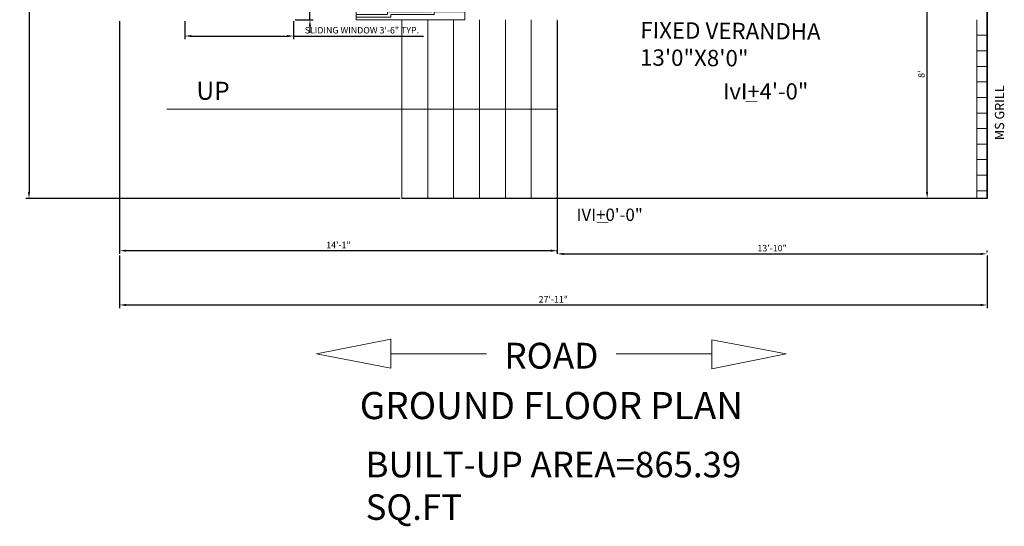
# Model space of a CAD drawing. Units: inches. Extents: x 918 to 1328, y 603 to 1174.
# Tile 1 of 4: x 918 to 1298, y 603 to 798. Entities that reach past the tile are written whole.
import ezdxf

# ---------------------------------------------------------------- set-up
doc = ezdxf.new("R2010")
doc.units = ezdxf.units.IN
for name, color, linetype, lineweight in [('A-ANNO-DIMS', 1, 'Continuous', 18), ('A-ANNO-SYMB', 1, 'Continuous', 18), ('A-ANNO-TEXT', 7, 'Continuous', 18), ('A-ANNO-TITL', 7, 'Continuous', 25), ('A-FLOR', 7, 'Continuous', 25), ('A-FLOR-RAIL', 7, 'Continuous', 18), ('A-GLAZ', 4, 'Continuous', 18), ('A-WALL', 7, 'Continuous', 35)]:
    doc.layers.add(name, color=color, linetype=linetype, lineweight=lineweight)
doc.layers.add('A-AREA-IDEN', color=251, linetype='Continuous', lineweight=20, true_color=0x636466)
doc.layers.add('A-FLOR-STRS', color=251, linetype='Continuous', lineweight=20, true_color=0x636466)
doc.styles.get("Standard").update_dxf_attribs({"font": 'arial.ttf'})
doc.dimstyles.new('ISO-25', dxfattribs={"dimtxt": 2.5, "dimasz": 2.5, "dimexe": 1.25, "dimexo": 0.625, "dimtad": 1, "dimdec": 0, "dimlunit": 3, "dimtxsty": 'Standard', "dimcen": 2.5, "dimadec": 0, "dimazin": 0, "dimtfac": 1, "dimtdec": 0, "dimtmove": 0, "dimatfit": 3, "dimfxl": 1, "dimarcsym": 0})

# ---------------------------------------------------------------- blocks, each defined once
blk = doc.blocks.new('*D11')
at = {"layer": 'A-ANNO-DIMS', "color": 0, "lineweight": -2, "transparency": 16777216}
for p, q in [((956.48, 797.62), (956.48, 707.87)), ((1125.48, 797.62), (1125.48, 707.87)), ((958.98, 709.12), (1122.98, 709.12))]:
    blk.add_line(p, q, dxfattribs=at)
at = {"layer": 'A-ANNO-DIMS', "color": 0, "transparency": 16777216}
for points in [[(958.98, 709.53), (958.98, 708.7), (956.48, 709.12)], [(1122.98, 709.53), (1122.98, 708.7), (1125.48, 709.12)]]:
    blk.add_solid(points, dxfattribs=at)
at = {"layer": 'Defpoints', "color": 0, "transparency": 16777216}
for p in [(956.48, 798.24), (1125.48, 798.24), (1125.48, 709.12)]:
    blk.add_point(p, dxfattribs=at)
at = {"layer": 'A-ANNO-DIMS', "color": 0, "transparency": 16777216, "insert": (1040.98, 711), "char_height": 2.5, "attachment_point": 5}
blk.add_mtext('14\'-1"', dxfattribs=at)
blk = doc.blocks.new('*D19')
at = {"layer": 'A-ANNO-DIMS', "color": 0, "lineweight": -2, "transparency": 16777216}
for p, q in [((956.48, 707.24), (956.48, 686.91)), ((1291.48, 707.24), (1291.48, 686.91)), ((958.98, 688.16), (1288.98, 688.16))]:
    blk.add_line(p, q, dxfattribs=at)
at = {"layer": 'A-ANNO-DIMS', "color": 0, "transparency": 16777216}
for points in [[(958.98, 688.58), (958.98, 687.74), (956.48, 688.16)], [(1288.98, 688.58), (1288.98, 687.74), (1291.48, 688.16)]]:
    blk.add_solid(points, dxfattribs=at)
at = {"layer": 'Defpoints', "color": 0, "transparency": 16777216}
for p in [(956.48, 707.87), (1291.48, 707.87), (1291.48, 688.16)]:
    blk.add_point(p, dxfattribs=at)
at = {"layer": 'A-ANNO-DIMS', "color": 0, "transparency": 16777216, "insert": (1123.98, 690.04), "char_height": 2.5, "attachment_point": 5}
blk.add_mtext('27\'-11"', dxfattribs=at)
blk = doc.blocks.new('*D20')
at = {"layer": 'A-ANNO-DIMS', "color": 0, "lineweight": -2, "transparency": 16777216}
for p, q in [((1272.05, 825.24), (1267.09, 825.24)), ((1268.34, 731.74), (1268.34, 822.74)), ((1272.05, 729.24), (1267.09, 729.24))]:
    blk.add_line(p, q, dxfattribs=at)
at = {"layer": 'A-ANNO-DIMS', "color": 0, "transparency": 16777216}
for points in [[(1267.92, 822.74), (1268.75, 822.74), (1268.34, 825.24)], [(1267.92, 731.74), (1268.75, 731.74), (1268.34, 729.24)]]:
    blk.add_solid(points, dxfattribs=at)
at = {"layer": 'Defpoints', "color": 0, "transparency": 16777216}
for p in [(1268.34, 825.24), (1272.68, 825.24), (1272.68, 729.24)]:
    blk.add_point(p, dxfattribs=at)
at = {"layer": 'A-ANNO-DIMS', "color": 0, "transparency": 16777216, "insert": (1266.44, 777.24), "char_height": 2.5, "attachment_point": 5, "rotation": 90}
blk.add_mtext("8'", dxfattribs=at)
blk = doc.blocks.new('*D21')
at = {"layer": 'A-ANNO-DIMS', "color": 0, "lineweight": -2, "transparency": 16777216}
for p, q in [((1125.48, 708.49), (1125.48, 709.12)), ((1127.98, 707.87), (1288.98, 707.87)), ((1291.48, 708.49), (1291.48, 709.12))]:
    blk.add_line(p, q, dxfattribs=at)
at = {"layer": 'A-ANNO-DIMS', "color": 0, "transparency": 16777216}
for points in [[(1127.98, 708.28), (1127.98, 707.45), (1125.48, 707.87)], [(1288.98, 708.28), (1288.98, 707.45), (1291.48, 707.87)]]:
    blk.add_solid(points, dxfattribs=at)
at = {"layer": 'Defpoints', "color": 0, "transparency": 16777216}
for p in [(1125.48, 707.87), (1291.48, 707.87), (1291.48, 707.87)]:
    blk.add_point(p, dxfattribs=at)
at = {"layer": 'A-ANNO-DIMS', "color": 0, "transparency": 16777216, "insert": (1208.48, 709.77), "char_height": 2.5, "attachment_point": 5}
blk.add_mtext('13\'-10"', dxfattribs=at)
blk = doc.blocks.new('WIN-SLIDING-42')
for p, q in [((0, 5), (0, 0)), ((42, 5), (0, 5)), ((29.09, 3), (29.09, 4.02)), ((29.09, 4.02), (42, 4.02)), ((42, 0), (42, 5)), ((0, 1.97), (12.14, 1.97)), ((0, 0.97), (13.35, 0.97)), ((0, 0), (42, 0)), ((12.14, 3), (29.09, 3)), ((12.14, 1.97), (12.14, 3)), ((13.35, 0.97), (13.35, 1.97)), ((13.35, 1.97), (30.11, 1.97)), ((30.11, 1.97), (30.11, 3)), ((30.11, 3), (42, 3))]:
    blk.add_line(p, q)
blk = doc.blocks.new('ARROW-ROAD')
for p, q in [((65.62, 5.76), (36.95, 11.23)), ((36.95, 11.23), (36.95, 0)), ((0, 5.76), (36.95, 5.76)), ((36.95, 0), (65.62, 5.76))]:
    blk.add_line(p, q)
blk = doc.blocks.new('*D32')
at = {"layer": 'A-ANNO-DIMS', "color": 0, "lineweight": -2, "transparency": 16777216}
for p, q in [((981.69, 797.62), (981.69, 790.69)), ((1023.69, 797.62), (1023.69, 790.69)), ((984.19, 791.94), (1021.19, 791.94)), ((1023.69, 791.94), (1073.9, 791.94))]:
    blk.add_line(p, q, dxfattribs=at)
at = {"layer": 'A-ANNO-DIMS', "color": 0, "transparency": 16777216}
for points in [[(984.19, 792.36), (984.19, 791.53), (981.69, 791.94)], [(1021.19, 792.36), (1021.19, 791.53), (1023.69, 791.94)]]:
    blk.add_solid(points, dxfattribs=at)
at = {"layer": 'Defpoints', "color": 0, "transparency": 16777216}
for p in [(981.69, 798.24), (1023.69, 798.24), (1023.69, 791.94)]:
    blk.add_point(p, dxfattribs=at)
at = {"layer": 'A-ANNO-DIMS', "color": 0, "transparency": 16777216, "insert": (1050.05, 793.86), "char_height": 2.5, "attachment_point": 5}
blk.add_mtext('SLIDING WINDOW 3\'-6" TYP.', dxfattribs=at)
blk = doc.blocks.new('*D33')
at = {"layer": 'A-ANNO-DIMS', "color": 0, "lineweight": -2, "transparency": 16777216}
for p, q in [((1029.99, 805.74), (1029.99, 824.73)), ((1024.31, 803.24), (1031.24, 803.24)), ((1029.99, 798.24), (1029.99, 803.24)), ((1024.31, 798.24), (1031.24, 798.24)), ((1029.99, 795.74), (1029.99, 793.24))]:
    blk.add_line(p, q, dxfattribs=at)
at = {"layer": 'A-ANNO-DIMS', "color": 0, "transparency": 16777216}
for points in [[(1029.57, 805.74), (1030.41, 805.74), (1029.99, 803.24)], [(1029.57, 795.74), (1030.41, 795.74), (1029.99, 798.24)]]:
    blk.add_solid(points, dxfattribs=at)
at = {"layer": 'Defpoints', "color": 0, "transparency": 16777216}
for p in [(1023.69, 803.24), (1029.99, 803.24), (1023.69, 798.24)]:
    blk.add_point(p, dxfattribs=at)
at = {"layer": 'A-ANNO-DIMS', "color": 0, "transparency": 16777216, "insert": (1028.09, 816.49), "char_height": 2.5, "attachment_point": 5, "rotation": 90}
blk.add_mtext('0\'-5" TYP.', dxfattribs=at)
blk = doc.blocks.new('*D44')
at = {"layer": 'A-ANNO-DIMS', "color": 0, "lineweight": -2, "transparency": 16777216}
for p, q in [((955.86, 1136.24), (920.25, 1136.24)), ((921.5, 1133.74), (921.5, 731.74)), ((1064.86, 729.24), (920.25, 729.24))]:
    blk.add_line(p, q, dxfattribs=at)
at = {"layer": 'A-ANNO-DIMS', "color": 0, "transparency": 16777216}
for points in [[(921.09, 1133.74), (921.92, 1133.74), (921.5, 1136.24)], [(921.09, 731.74), (921.92, 731.74), (921.5, 729.24)]]:
    blk.add_solid(points, dxfattribs=at)
at = {"layer": 'Defpoints', "color": 0, "transparency": 16777216}
for p in [(956.48, 1136.24), (921.5, 729.24), (1065.48, 729.24)]:
    blk.add_point(p, dxfattribs=at)
at = {"layer": 'A-ANNO-DIMS', "color": 0, "transparency": 16777216, "insert": (919.6, 932.74), "char_height": 2.5, "attachment_point": 5, "rotation": 90}
blk.add_mtext('33\'-11"', dxfattribs=at)

msp = doc.modelspace()

# ---------------------------------------------------------------- linework, layer by layer
at = {"layer": 'A-ANNO-SYMB'}
for p, q in [((1198.32, 766.78), (1202.69, 766.67)), ((1125.48, 763.74), (974.75, 763.74)), ((1140.75, 720.11), (1145.12, 720.01))]:
    msp.add_line(p, q, dxfattribs=at)
at = {"layer": 'A-FLOR'}
msp.add_line((1291.48, 729.24), (1065.48, 729.24), dxfattribs=at)
at = {"layer": 'A-FLOR-RAIL'}
for p, q in [((1287.48, 729.24), (1287.48, 798.24)), ((1287.48, 792.24), (1291.48, 792.24)), ((1287.48, 786.24), (1291.48, 786.24)), ((1287.48, 780.24), (1291.48, 780.24)), ((1287.48, 774.24), (1291.48, 774.24)), ((1287.48, 768.24), (1291.48, 768.24)), ((1287.48, 762.24), (1291.48, 762.24)), ((1287.48, 756.24), (1291.48, 756.24)), ((1287.48, 750.24), (1291.48, 750.24)), ((1287.48, 744.24), (1291.48, 744.24)), ((1287.48, 738.24), (1291.48, 738.24)), ((1287.48, 732.24), (1291.48, 732.24))]:
    msp.add_line(p, q, dxfattribs=at)
at = {"layer": 'A-FLOR-STRS'}
for p, q in [((1065.48, 798.24), (1065.48, 729.24)), ((1075.48, 798.24), (1075.48, 729.24)), ((1085.48, 798.24), (1085.48, 729.24)), ((1095.48, 798.24), (1095.48, 729.24)), ((1105.48, 798.24), (1105.48, 729.24)), ((1115.48, 798.24), (1115.48, 729.24)), ((1125.48, 798.24), (1125.48, 729.24))]:
    msp.add_line(p, q, dxfattribs=at)
at = {"layer": 'A-WALL'}
msp.add_line((1291.48, 729.24), (1291.48, 1136.24), dxfattribs=at)

# ---------------------------------------------------------------- block references
at = {"layer": 'A-ANNO-SYMB', "rotation": 180}
msp.add_blockref('ARROW-ROAD', (1098.17, 675.01), dxfattribs=at)
at = {"layer": 'A-ANNO-SYMB'}
msp.add_blockref('ARROW-ROAD', (1148.24, 663.5), dxfattribs=at)
at = {"layer": 'A-GLAZ'}
msp.add_blockref('WIN-SLIDING-42', (1047.83, 798.24), dxfattribs=at)

# ---------------------------------------------------------------- texts
at = {"layer": 'A-ANNO-SYMB', "attachment_point": 1}
for s, width, gutter_width, insert, char_height in [('IvI+4\'-0"', 50.3111, 31.19, (1189.51, 773.7), 6.237), ('IVI+0\'-0"', 24.2216, 23.91, (1132.94, 725.36), 4.782)]:
    msp.add_mtext_dynamic_manual_height_columns(s, width=width, gutter_width=gutter_width, heights=[0], dxfattribs=dict(at, insert=insert, char_height=char_height))
at = {"layer": 'A-ANNO-TEXT', "attachment_point": 1}
for s, width, gutter_width, insert, char_height in [('UP', 49.361, 34.85, (986.13, 774.29), 6.97), ('ROAD', 149.2838, 49.82, (1105.07, 673.57), 9.963)]:
    msp.add_mtext_dynamic_manual_height_columns(s, width=width, gutter_width=gutter_width, heights=[0], dxfattribs=dict(at, insert=insert, char_height=char_height))
at = {"layer": 'A-ANNO-TEXT', "insert": (1294.52, 751.78), "char_height": 3.569, "attachment_point": 1, "rotation": 90}
msp.add_mtext_dynamic_manual_height_columns('MS GRILL', width=23.044, gutter_width=17.85, heights=[0], dxfattribs=at)
at = {"layer": 'A-ANNO-TITL', "attachment_point": 1}
for s, width, gutter_width, insert, char_height in [('GROUND FLOOR PLAN', 269.0949, 52.32, (1049.23, 654.58), 10.4646), ('BUILT-UP AREA=865.39 SQ.FT', 166.9665, 49.28, (1051.5, 631.52), 9.8569)]:
    msp.add_mtext_dynamic_manual_height_columns(s, width=width, gutter_width=gutter_width, heights=[0], dxfattribs=dict(at, insert=insert, char_height=char_height))
at = {"layer": 'A-AREA-IDEN', "insert": (1157.59, 797.39), "char_height": 6.324, "attachment_point": 1, "rotation": 359.5323}
msp.add_mtext_dynamic_manual_height_columns('FIXED VERANDHA\\P13\'0"X8\'0"', width=282.3955, gutter_width=66.56, heights=[0], dxfattribs=at)

# ---------------------------------------------------------------- dimensions: what is measured, and where the dimension line sits
at = {"layer": 'A-ANNO-DIMS'}
for base, p1, p2, override, picture, middle in [((921.5, 729.24), (956.48, 1136.24), (1065.48, 729.24), {"dimdec": 1, "dimlfac": 1, "dimrnd": 0, "dimzin": 1, "dimdsep": 46, "dimlunit": 4, "dimfrac": 2}, '*D44', (919.6, 932.74)), ((1268.34, 825.24), (1272.68, 729.24), (1272.68, 825.24), {"dimclrd": 0, "dimclre": 0, "dimclrt": 0}, '*D20', (1266.44, 777.24))]:
    dim = msp.add_linear_dim(base=base, p1=p1, p2=p2, angle=90, dimstyle='ISO-25', override=override, dxfattribs=at)
    dim.commit()
    dim.dimension.update_dxf_attribs({"geometry": picture, "text_midpoint": middle})
dim = msp.add_linear_dim(base=(1029.99, 803.24), p1=(1023.69, 798.24), p2=(1023.69, 803.24), angle=90, text='<> TYP.', dimstyle='ISO-25', override={"dimdec": 1, "dimlfac": 1, "dimrnd": 0, "dimzin": 1, "dimdsep": 46, "dimlunit": 4, "dimfrac": 2}, dxfattribs=at)
dim.commit()
dim.dimension.update_dxf_attribs({"geometry": '*D33', "text_midpoint": (1028.09, 816.49)})
dim = msp.add_linear_dim(base=(1023.69, 791.94), p1=(981.69, 798.24), p2=(1023.69, 798.24), text='SLIDING WINDOW <> TYP.', dimstyle='ISO-25', override={"dimdec": 1, "dimlfac": 1, "dimrnd": 0, "dimzin": 1, "dimdsep": 46, "dimlunit": 4, "dimfrac": 2}, dxfattribs=at)
dim.commit()
dim.dimension.update_dxf_attribs({"geometry": '*D32', "text_midpoint": (1050.05, 793.86)})
for base, p1, p2, picture, middle in [((1125.48, 709.12), (956.48, 798.24), (1125.48, 798.24), '*D11', (1040.98, 711)), ((1291.48, 707.87), (1125.48, 707.87), (1291.48, 707.87), '*D21', (1208.48, 709.77)), ((1291.48, 688.16), (956.48, 707.87), (1291.48, 707.87), '*D19', (1123.98, 690.04))]:
    dim = msp.add_linear_dim(base=base, p1=p1, p2=p2, dimstyle='ISO-25', override={"dimclrd": 0, "dimclre": 0, "dimclrt": 0}, dxfattribs=at)
    dim.commit()
    dim.dimension.update_dxf_attribs({"geometry": picture, "text_midpoint": middle})

doc.saveas('drawing.dxf')
